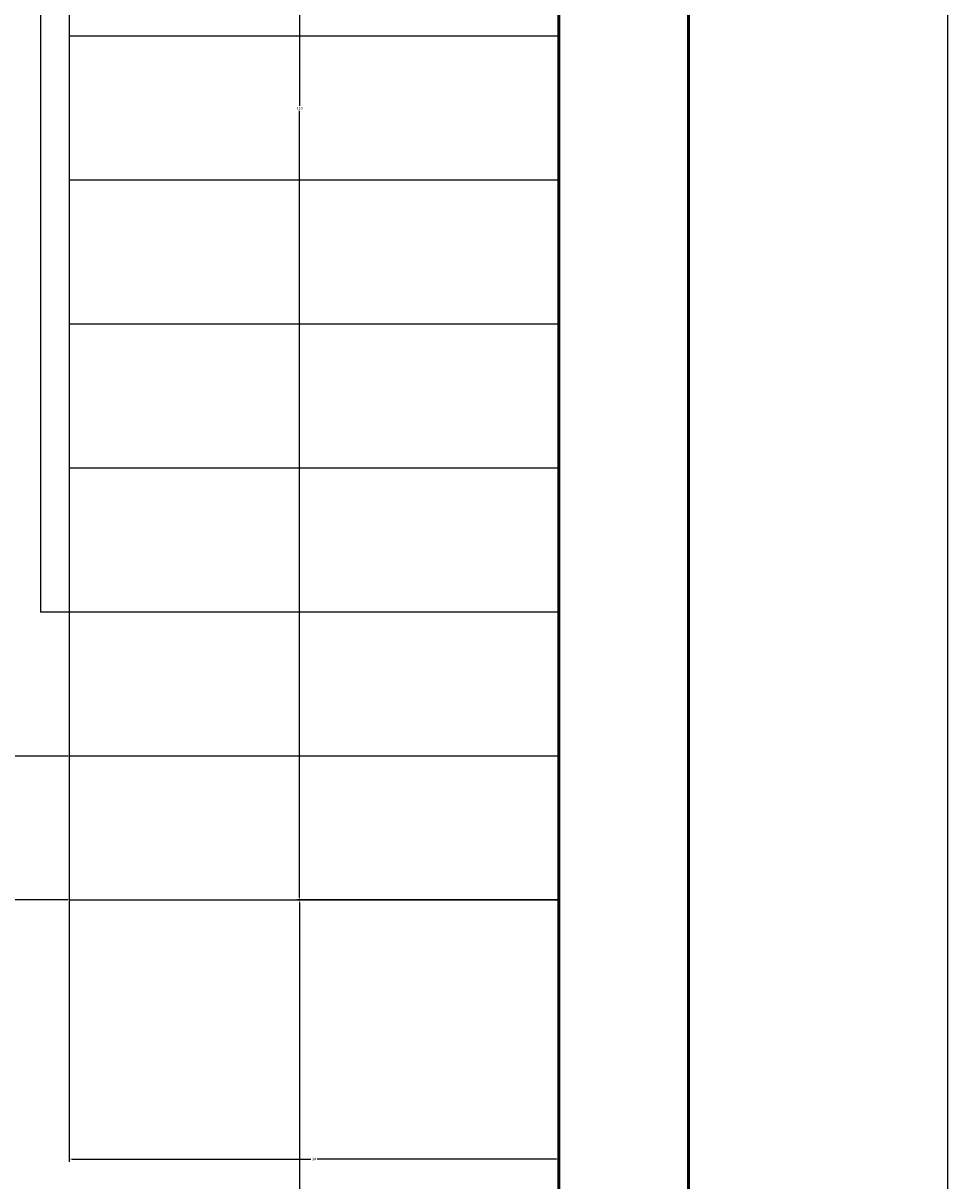
# Model space of a CAD drawing. Units: inches. Extents: x 2621 to 2849, y 2066 to 2463.
# Tile 6 of 28: x 2785 to 2849, y 2119 to 2199. Entities that reach past the tile are written whole.
import ezdxf

# ---------------------------------------------------------------- set-up
doc = ezdxf.new("R2010")
doc.units = ezdxf.units.IN
for name, color, linetype, lineweight in [('A-ANNO-DIMS', 2, 'Continuous', 18), ('A-FLOR-STRS', 7, 'Continuous', 25), ('A-WALL', 7, 'Continuous', 50)]:
    doc.layers.add(name, color=color, linetype=linetype, lineweight=lineweight)
doc.styles.get("Standard").update_dxf_attribs({"font": 'arial.ttf'})
doc.dimstyles.get("Standard").update_dxf_attribs({"dimtxt": 0.18, "dimasz": 0.18, "dimexe": 0.18, "dimexo": 0.0625, "dimgap": 0.09, "dimtad": 0, "dimtih": 1, "dimtoh": 1, "dimdec": 4, "dimzin": 0, "dimdsep": 46, "dimtxsty": 'Standard', "dimcen": 0.09, "dimadec": 0, "dimazin": 0, "dimtfac": 1, "dimtdec": 4, "dimtofl": 0, "dimtmove": 0, "dimatfit": 3, "dimfxl": 1, "dimtolj": 1, "dimtzin": 0, "dimarcsym": 0})

# ---------------------------------------------------------------- blocks, each defined once
blk = doc.blocks.new('*D36')
at = {"layer": 'A-ANNO-DIMS', "color": 0, "lineweight": -2, "transparency": 16777216}
for p, q in [((2830.933, 2444.375), (2849.054, 2444.375)), ((2848.874, 2444.195), (2848.874, 2264.557)), ((2848.874, 2084.555), (2848.874, 2264.193)), ((2830.933, 2084.375), (2849.054, 2084.375))]:
    blk.add_line(p, q, dxfattribs=at)
at = {"layer": 'A-ANNO-DIMS', "color": 0, "transparency": 16777216}
for points in [[(2848.844, 2444.195), (2848.904, 2444.195), (2848.874, 2444.375)], [(2848.844, 2084.555), (2848.904, 2084.555), (2848.874, 2084.375)]]:
    blk.add_solid(points, dxfattribs=at)
at = {"layer": 'Defpoints', "color": 0, "transparency": 16777216}
for p in [(2830.87, 2444.375), (2848.874, 2444.375), (2830.87, 2084.375)]:
    blk.add_point(p, dxfattribs=at)
at = {"layer": 'A-ANNO-DIMS', "color": 0, "transparency": 16777216, "insert": (2848.874, 2264.375), "char_height": 0.18, "attachment_point": 5}
blk.add_mtext('\\A1;360', dxfattribs=at)
blk = doc.blocks.new('*D58')
at = {"layer": 'A-ANNO-DIMS', "color": 0, "lineweight": -2, "transparency": 16777216}
for p, q in [((2821.808, 2248.46), (2803.687, 2248.46)), ((2803.867, 2248.28), (2803.867, 2193.642)), ((2803.867, 2138.64), (2803.867, 2193.278)), ((2821.808, 2138.46), (2803.687, 2138.46))]:
    blk.add_line(p, q, dxfattribs=at)
at = {"layer": 'A-ANNO-DIMS', "color": 0, "transparency": 16777216}
for points in [[(2803.837, 2248.28), (2803.897, 2248.28), (2803.867, 2248.46)], [(2803.837, 2138.64), (2803.897, 2138.64), (2803.867, 2138.46)]]:
    blk.add_solid(points, dxfattribs=at)
at = {"layer": 'Defpoints', "color": 0, "transparency": 16777216}
for p in [(2803.867, 2248.46), (2821.87, 2248.46), (2821.87, 2138.46)]:
    blk.add_point(p, dxfattribs=at)
at = {"layer": 'A-ANNO-DIMS', "color": 0, "transparency": 16777216, "insert": (2803.867, 2193.46), "char_height": 0.18, "attachment_point": 5}
blk.add_mtext('\\A1;110', dxfattribs=at)
blk = doc.blocks.new('*D59')
at = {"layer": 'A-ANNO-DIMS', "color": 0, "lineweight": -2, "transparency": 16777216}
for p, q in [((2787.87, 2138.397), (2787.87, 2120.276)), ((2821.87, 2138.397), (2821.87, 2120.276)), ((2788.05, 2120.456), (2804.652, 2120.456)), ((2821.69, 2120.456), (2805.089, 2120.456))]:
    blk.add_line(p, q, dxfattribs=at)
at = {"layer": 'A-ANNO-DIMS', "color": 0, "transparency": 16777216}
for points in [[(2788.05, 2120.486), (2788.05, 2120.426), (2787.87, 2120.456)], [(2821.69, 2120.486), (2821.69, 2120.426), (2821.87, 2120.456)]]:
    blk.add_solid(points, dxfattribs=at)
at = {"layer": 'Defpoints', "color": 0, "transparency": 16777216}
for p in [(2787.87, 2138.46), (2821.87, 2138.46), (2787.87, 2120.456)]:
    blk.add_point(p, dxfattribs=at)
at = {"layer": 'A-ANNO-DIMS', "color": 0, "transparency": 16777216, "insert": (2804.87, 2120.456), "char_height": 0.18, "attachment_point": 5}
blk.add_mtext('\\A1;34', dxfattribs=at)
blk = doc.blocks.new('*D60')
at = {"layer": 'A-ANNO-DIMS', "color": 0, "lineweight": -2, "transparency": 16777216}
for p, q in [((2821.808, 2138.46), (2803.687, 2138.46)), ((2803.867, 2138.28), (2803.867, 2116.099)), ((2803.867, 2093.555), (2803.867, 2115.735)), ((2821.808, 2093.375), (2803.687, 2093.375))]:
    blk.add_line(p, q, dxfattribs=at)
at = {"layer": 'A-ANNO-DIMS', "color": 0, "transparency": 16777216}
for points in [[(2803.837, 2138.28), (2803.897, 2138.28), (2803.867, 2138.46)], [(2803.837, 2093.555), (2803.897, 2093.555), (2803.867, 2093.375)]]:
    blk.add_solid(points, dxfattribs=at)
at = {"layer": 'Defpoints', "color": 0, "transparency": 16777216}
for p in [(2803.867, 2138.46), (2821.87, 2138.46), (2821.87, 2093.375)]:
    blk.add_point(p, dxfattribs=at)
at = {"layer": 'A-ANNO-DIMS', "color": 0, "transparency": 16777216, "insert": (2803.867, 2115.917), "char_height": 0.18, "attachment_point": 5}
blk.add_mtext('\\A1;45.085', dxfattribs=at)
blk = doc.blocks.new('*D61')
at = {"layer": 'A-ANNO-DIMS', "color": 0, "lineweight": -2, "transparency": 16777216}
for p, q in [((2787.808, 2148.46), (2769.687, 2148.46)), ((2769.867, 2148.28), (2769.867, 2143.642)), ((2769.867, 2138.64), (2769.867, 2143.278)), ((2787.808, 2138.46), (2769.687, 2138.46))]:
    blk.add_line(p, q, dxfattribs=at)
at = {"layer": 'A-ANNO-DIMS', "color": 0, "transparency": 16777216}
for points in [[(2769.837, 2148.28), (2769.897, 2148.28), (2769.867, 2148.46)], [(2769.837, 2138.64), (2769.897, 2138.64), (2769.867, 2138.46)]]:
    blk.add_solid(points, dxfattribs=at)
at = {"layer": 'Defpoints', "color": 0, "transparency": 16777216}
for p in [(2769.867, 2148.46), (2787.87, 2148.46), (2787.87, 2138.46)]:
    blk.add_point(p, dxfattribs=at)
at = {"layer": 'A-ANNO-DIMS', "color": 0, "transparency": 16777216, "insert": (2769.867, 2143.46), "char_height": 0.18, "attachment_point": 5}
blk.add_mtext('\\A1;10', dxfattribs=at)

msp = doc.modelspace()

# ---------------------------------------------------------------- linework, layer by layer
at = {"layer": 'A-FLOR-STRS'}
for p, q in [((2785.8701, 2248.4598), (2785.8701, 2158.4598)), ((2787.8701, 2248.4598), (2787.8701, 2158.4598)), ((2821.8701, 2198.4598), (2787.8701, 2198.4598)), ((2821.8701, 2188.4598), (2787.8701, 2188.4598)), ((2821.8701, 2178.4598), (2787.8701, 2178.4598)), ((2821.8701, 2168.4598), (2787.8701, 2168.4598)), ((2821.8701, 2158.4598), (2785.8701, 2158.4598)), ((2787.8701, 2158.4598), (2787.8701, 2138.4598)), ((2821.8701, 2148.4598), (2787.8701, 2148.4598)), ((2787.8701, 2138.4598), (2821.8701, 2138.4598))]:
    msp.add_line(p, q, dxfattribs=at)
at = {"layer": 'A-WALL'}
msp.add_line((2821.8701, 2371.3746), (2821.8701, 2093.3746), dxfattribs=at)
msp.add_lwpolyline([(2761.8701, 2084.3746), (2638.8701, 2084.3746), (2638.8701, 2444.3746), (2830.8701, 2444.3746), (2830.8701, 2084.3746), (2797.8701, 2084.3746)], dxfattribs=at)

# ---------------------------------------------------------------- dimensions: what is measured, and where the dimension line sits
at = {"layer": 'A-ANNO-DIMS'}
for base, p1, p2, angle, override, picture, middle in [((2848.8736, 2444.3746), (2830.8701, 2084.3746), (2830.8701, 2444.3746), 90, {"dimdec": 0, "dimlfac": 1, "dimrnd": 0, "dimzin": 0, "dimdsep": 46, "dimlunit": 2}, '*D36', (2848.8736, 2264.3746)), ((2803.8666, 2248.4598), (2821.8701, 2138.4598), (2821.8701, 2248.4598), 90, {"dimdec": 0, "dimlfac": 1, "dimrnd": 0, "dimzin": 0, "dimdsep": 46, "dimlunit": 2}, '*D58', (2803.8666, 2193.4598)), ((2769.8666, 2148.4598), (2787.8701, 2138.4598), (2787.8701, 2148.4598), 90, {"dimdec": 0, "dimlfac": 1, "dimrnd": 0, "dimzin": 0, "dimdsep": 46, "dimlunit": 2}, '*D61', (2769.8666, 2143.4598)), ((2787.8701, 2120.4563), (2821.8701, 2138.4598), (2787.8701, 2138.4598), 180, {"dimdec": 0, "dimlfac": 1, "dimrnd": 0, "dimzin": 0, "dimdsep": 46, "dimlunit": 2}, '*D59', (2804.8701, 2120.4563)), ((2803.8666, 2138.4598), (2821.8701, 2093.3746), (2821.8701, 2138.4598), 90, {"dimdec": 3, "dimlfac": 1, "dimrnd": 0, "dimzin": 0, "dimdsep": 46, "dimlunit": 2}, '*D60', (2803.8666, 2115.9172))]:
    dim = msp.add_linear_dim(base=base, p1=p1, p2=p2, angle=angle, dimstyle='Standard', override=override, dxfattribs=at)
    dim.commit()
    dim.dimension.update_dxf_attribs({"geometry": picture, "text_midpoint": middle})

doc.saveas('drawing.dxf')
